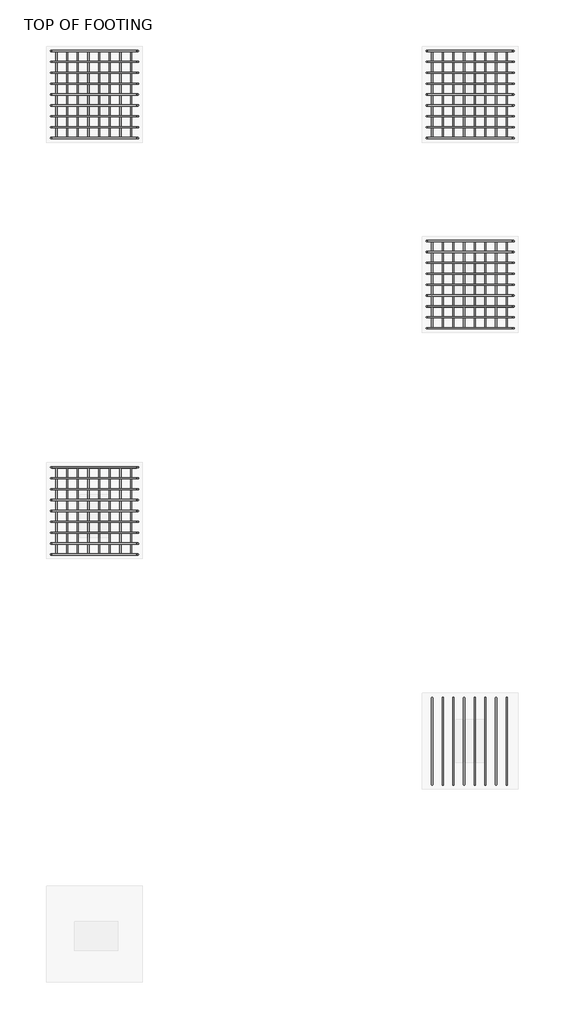
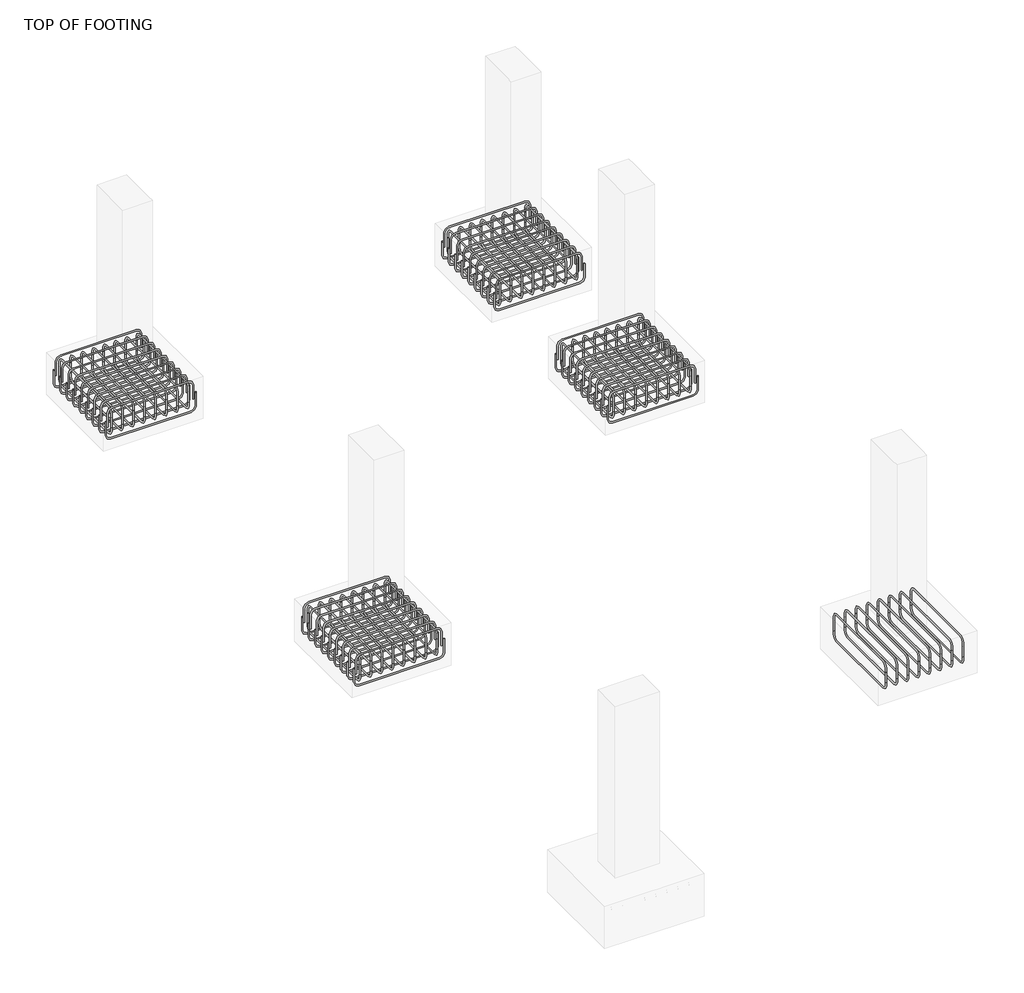
# One storey, part 12 of 20: 18 reinforcing bars.
"""IFC4 building model written with IfcOpenShell, lengths in millimetres."""

from ifc_helpers import new_model, si_unit, point, frame, origin, place, context, project, spatial, polyline, circle_curve, trimmed, segment, composite_curve, source, transform, mapped, element, save
from ifc_brep_helpers import swept_disk

model = new_model("IFC4")

# Units and contexts
model_context = context("Model", 3, world=origin())
ifc_project = project(units=[si_unit("LENGTHUNIT", "METRE", prefix="MILLI")], contexts=[model_context])

# Site, building, storey
site = spatial("IfcSite", under=ifc_project)
building = spatial("IfcBuilding", under=site)
storey = spatial("IfcBuildingStorey", under=building, Name="TOP OF FOOTING", Elevation=-1828.8)

# Reinforcing bars
placement = place(None, origin())
reinforcing_bar_shape = source(origin(), model_context, "Body", "SolidModel", [
    swept_disk(composite_curve([segment(polyline([(-5285.1605653, 14441.1679708, -2006.6587682), (-5285.1605653, 14441.1679708, -2153.9587682)]), True, "CONTINUOUS"), segment(trimmed(circle_curve(frame((-5331.5105653, 14441.1679708, -2153.9587682), z_axis=(0.0, 1.0, 0.0), x_axis=(46.350000000000364, 0.0, 0.0)), 46.35), [point((-5285.1605653, 14441.1679708, -2153.9587682))], [point((-5331.5105653, 14441.1679708, -2200.3087682))], True, "CARTESIAN"), True, "CONTINUOUS"), segment(polyline([(-5331.5105653, 14441.1679708, -2200.3087682), (-6146.1105653, 14441.1679708, -2200.3087682)]), True, "CONTINUOUS"), segment(trimmed(circle_curve(frame((-6146.1105653, 14441.1679708, -2153.9587682), z_axis=(0.0, 1.0, 0.0), x_axis=(0.0, 0.0, -46.34999999999991)), 46.35), [point((-6146.1105653, 14441.1679708, -2200.3087682))], [point((-6192.4605653, 14441.1679708, -2153.9587682))], True, "CARTESIAN"), True, "CONTINUOUS"), segment(polyline([(-6192.4605653, 14441.1679708, -2153.9587682), (-6192.4605653, 14441.1679708, -2006.6587682)]), True, "CONTINUOUS")], self_intersect=False), 6.35),
])
element("IfcReinforcingBar", 1, at=placement, inside=storey, context=model_context, shape_type="MappedRepresentation", body=[
    mapped(reinforcing_bar_shape, transform((0.0, 0.0, 0.0), x_axis=(1.0, 0.0, 0.0), y_axis=(0.0, 1.0, 0.0), z_axis=(0.0, 0.0, 1.0))),
    mapped(reinforcing_bar_shape, transform((0.0, -113.4125, 0.0), x_axis=(1.0, 0.0, 0.0), y_axis=(0.0, 1.0, 0.0), z_axis=(0.0, 0.0, 1.0))),
    mapped(reinforcing_bar_shape, transform((0.0, -226.825, 0.0), x_axis=(1.0, 0.0, 0.0), y_axis=(0.0, 1.0, 0.0), z_axis=(0.0, 0.0, 1.0))),
    mapped(reinforcing_bar_shape, transform((0.0, -340.2375, 0.0), x_axis=(1.0, 0.0, 0.0), y_axis=(0.0, 1.0, 0.0), z_axis=(0.0, 0.0, 1.0))),
    mapped(reinforcing_bar_shape, transform((0.0, -453.65, 0.0), x_axis=(1.0, 0.0, 0.0), y_axis=(0.0, 1.0, 0.0), z_axis=(0.0, 0.0, 1.0))),
    mapped(reinforcing_bar_shape, transform((0.0, -567.0625, 0.0), x_axis=(1.0, 0.0, 0.0), y_axis=(0.0, 1.0, 0.0), z_axis=(0.0, 0.0, 1.0))),
    mapped(reinforcing_bar_shape, transform((0.0, -680.475, 0.0), x_axis=(1.0, 0.0, 0.0), y_axis=(0.0, 1.0, 0.0), z_axis=(0.0, 0.0, 1.0))),
    mapped(reinforcing_bar_shape, transform((0.0, -793.8875, 0.0), x_axis=(1.0, 0.0, 0.0), y_axis=(0.0, 1.0, 0.0), z_axis=(0.0, 0.0, 1.0))),
    mapped(reinforcing_bar_shape, transform((0.0, -907.3, 0.0), x_axis=(1.0, 0.0, 0.0), y_axis=(0.0, 1.0, 0.0), z_axis=(0.0, 0.0, 1.0))),
])
reinforcing_bar_2_shape = source(origin(), model_context, "Body", "SolidModel", [
    swept_disk(composite_curve([segment(polyline([(-6172.986454, 14441.1679708, -2068.8), (-6172.986454, 14441.1679708, -1921.5)]), True, "CONTINUOUS"), segment(trimmed(circle_curve(frame((-6126.636454, 14441.1679708, -1921.5), z_axis=(0.0, 1.0, 0.0), x_axis=(-46.349999999999454, 0.0, 0.0)), 46.35), [point((-6172.986454, 14441.1679708, -1921.5))], [point((-6126.636454, 14441.1679708, -1875.15))], True, "CARTESIAN"), True, "CONTINUOUS"), segment(polyline([(-6126.636454, 14441.1679708, -1875.15), (-5357.1730543, 14441.1679708, -1875.15)]), True, "CONTINUOUS"), segment(trimmed(circle_curve(frame((-5357.1730543, 14441.1679708, -1921.5), z_axis=(0.0, 1.0, 0.0), x_axis=(0.0, 0.0, 46.34999999999991)), 46.35), [point((-5357.1730543, 14441.1679708, -1875.15))], [point((-5310.8230543, 14441.1679708, -1921.5))], True, "CARTESIAN"), True, "CONTINUOUS"), segment(polyline([(-5310.8230543, 14441.1679708, -1921.5), (-5310.8230543, 14441.1679708, -2068.8)]), True, "CONTINUOUS")], self_intersect=False), 6.35),
])
element("IfcReinforcingBar", 2, at=placement, inside=storey, context=model_context, shape_type="MappedRepresentation", body=[
    mapped(reinforcing_bar_2_shape, transform((0.0, 0.0, 0.0), x_axis=(1.0, 0.0, 0.0), y_axis=(0.0, 1.0, 0.0), z_axis=(0.0, 0.0, 1.0))),
    mapped(reinforcing_bar_2_shape, transform((0.0, -113.4125, 0.0), x_axis=(1.0, 0.0, 0.0), y_axis=(0.0, 1.0, 0.0), z_axis=(0.0, 0.0, 1.0))),
    mapped(reinforcing_bar_2_shape, transform((0.0, -226.825, 0.0), x_axis=(1.0, 0.0, 0.0), y_axis=(0.0, 1.0, 0.0), z_axis=(0.0, 0.0, 1.0))),
    mapped(reinforcing_bar_2_shape, transform((0.0, -340.2375, 0.0), x_axis=(1.0, 0.0, 0.0), y_axis=(0.0, 1.0, 0.0), z_axis=(0.0, 0.0, 1.0))),
    mapped(reinforcing_bar_2_shape, transform((0.0, -453.65, 0.0), x_axis=(1.0, 0.0, 0.0), y_axis=(0.0, 1.0, 0.0), z_axis=(0.0, 0.0, 1.0))),
    mapped(reinforcing_bar_2_shape, transform((0.0, -567.0625, 0.0), x_axis=(1.0, 0.0, 0.0), y_axis=(0.0, 1.0, 0.0), z_axis=(0.0, 0.0, 1.0))),
    mapped(reinforcing_bar_2_shape, transform((0.0, -680.475, 0.0), x_axis=(1.0, 0.0, 0.0), y_axis=(0.0, 1.0, 0.0), z_axis=(0.0, 0.0, 1.0))),
    mapped(reinforcing_bar_2_shape, transform((0.0, -793.8875, 0.0), x_axis=(1.0, 0.0, 0.0), y_axis=(0.0, 1.0, 0.0), z_axis=(0.0, 0.0, 1.0))),
    mapped(reinforcing_bar_2_shape, transform((0.0, -907.3, 0.0), x_axis=(1.0, 0.0, 0.0), y_axis=(0.0, 1.0, 0.0), z_axis=(0.0, 0.0, 1.0))),
])
reinforcing_bar_3_shape = source(origin(), model_context, "Body", "SolidModel", [
    swept_disk(composite_curve([segment(polyline([(-5356.6575267, 14441.1679708, -2086.1951968), (-5356.6575267, 14441.1679708, -1938.8951968)]), True, "CONTINUOUS"), segment(trimmed(circle_curve(frame((-5356.6575267, 14394.8179708, -1938.8951968), z_axis=(1.0, 0.0, 0.0), x_axis=(0.0, 46.349999999998545, 0.0)), 46.35), [point((-5356.6575267, 14441.1679708, -1938.8951968))], [point((-5356.6575267, 14394.8179708, -1892.5451968))], True, "CARTESIAN"), True, "CONTINUOUS"), segment(polyline([(-5356.6575267, 14394.8179708, -1892.5451968), (-5356.6575267, 13580.2179708, -1892.5451968)]), True, "CONTINUOUS"), segment(trimmed(circle_curve(frame((-5356.6575267, 13580.2179708, -1938.8951968), z_axis=(1.0, 0.0, 0.0), x_axis=(0.0, 0.0, 46.34999999999991)), 46.35), [point((-5356.6575267, 13580.2179708, -1892.5451968))], [point((-5356.6575267, 13533.8679708, -1938.8951968))], True, "CARTESIAN"), True, "CONTINUOUS"), segment(polyline([(-5356.6575267, 13533.8679708, -1938.8951968), (-5356.6575267, 13533.8679708, -2086.1951968)]), True, "CONTINUOUS")], self_intersect=False), 6.35),
])
element("IfcReinforcingBar", 3, at=placement, inside=storey, context=model_context, shape_type="MappedRepresentation", body=[
    mapped(reinforcing_bar_3_shape, transform((0.0, 0.0, 0.0), x_axis=(1.0, 0.0, 0.0), y_axis=(0.0, 1.0, 0.0), z_axis=(0.0, 0.0, 1.0))),
    mapped(reinforcing_bar_3_shape, transform((-111.2862402, 0.0, 0.0), x_axis=(1.0, 0.0, 0.0), y_axis=(0.0, 1.0, 0.0), z_axis=(0.0, 0.0, 1.0))),
    mapped(reinforcing_bar_3_shape, transform((-222.5724804, 0.0, 0.0), x_axis=(1.0, 0.0, 0.0), y_axis=(0.0, 1.0, 0.0), z_axis=(0.0, 0.0, 1.0))),
    mapped(reinforcing_bar_3_shape, transform((-333.8587205, 0.0, 0.0), x_axis=(1.0, 0.0, 0.0), y_axis=(0.0, 1.0, 0.0), z_axis=(0.0, 0.0, 1.0))),
    mapped(reinforcing_bar_3_shape, transform((-445.1449607, 0.0, 0.0), x_axis=(1.0, 0.0, 0.0), y_axis=(0.0, 1.0, 0.0), z_axis=(0.0, 0.0, 1.0))),
    mapped(reinforcing_bar_3_shape, transform((-556.4312009, 0.0, 0.0), x_axis=(1.0, 0.0, 0.0), y_axis=(0.0, 1.0, 0.0), z_axis=(0.0, 0.0, 1.0))),
    mapped(reinforcing_bar_3_shape, transform((-667.7174411, 0.0, 0.0), x_axis=(1.0, 0.0, 0.0), y_axis=(0.0, 1.0, 0.0), z_axis=(0.0, 0.0, 1.0))),
    mapped(reinforcing_bar_3_shape, transform((-779.0036813, 0.0, 0.0), x_axis=(1.0, 0.0, 0.0), y_axis=(0.0, 1.0, 0.0), z_axis=(0.0, 0.0, 1.0))),
])
reinforcing_bar_4_shape = source(origin(), model_context, "Body", "SolidModel", [
    swept_disk(composite_curve([segment(polyline([(-6135.661208, 14441.1679708, -1979.1645013), (-6135.661208, 14441.1679708, -2126.4645013)]), True, "CONTINUOUS"), segment(trimmed(circle_curve(frame((-6135.661208, 14394.8179708, -2126.4645013), z_axis=(-1.0, 0.0, 0.0), x_axis=(0.0, 46.349999999998545, 0.0)), 46.35), [point((-6135.661208, 14441.1679708, -2126.4645013))], [point((-6135.661208, 14394.8179708, -2172.8145013))], True, "CARTESIAN"), True, "CONTINUOUS"), segment(polyline([(-6135.661208, 14394.8179708, -2172.8145013), (-6135.661208, 13580.2179708, -2172.8145013)]), True, "CONTINUOUS"), segment(trimmed(circle_curve(frame((-6135.661208, 13580.2179708, -2126.4645013), z_axis=(-1.0, 0.0, 0.0), x_axis=(0.0, 0.0, -46.34999999999991)), 46.35), [point((-6135.661208, 13580.2179708, -2172.8145013))], [point((-6135.661208, 13533.8679708, -2126.4645013))], True, "CARTESIAN"), True, "CONTINUOUS"), segment(polyline([(-6135.661208, 13533.8679708, -2126.4645013), (-6135.661208, 13533.8679708, -1979.1645013)]), True, "CONTINUOUS")], self_intersect=False), 6.35),
])
element("IfcReinforcingBar", 4, at=placement, inside=storey, context=model_context, shape_type="MappedRepresentation", body=[
    mapped(reinforcing_bar_4_shape, transform((0.0, 0.0, 0.0), x_axis=(1.0, 0.0, 0.0), y_axis=(0.0, 1.0, 0.0), z_axis=(0.0, 0.0, 1.0))),
    mapped(reinforcing_bar_4_shape, transform((111.2862402, 0.0, 0.0), x_axis=(1.0, 0.0, 0.0), y_axis=(0.0, 1.0, 0.0), z_axis=(0.0, 0.0, 1.0))),
    mapped(reinforcing_bar_4_shape, transform((222.5724804, 0.0, 0.0), x_axis=(1.0, 0.0, 0.0), y_axis=(0.0, 1.0, 0.0), z_axis=(0.0, 0.0, 1.0))),
    mapped(reinforcing_bar_4_shape, transform((333.8587205, 0.0, 0.0), x_axis=(1.0, 0.0, 0.0), y_axis=(0.0, 1.0, 0.0), z_axis=(0.0, 0.0, 1.0))),
    mapped(reinforcing_bar_4_shape, transform((445.1449607, 0.0, 0.0), x_axis=(1.0, 0.0, 0.0), y_axis=(0.0, 1.0, 0.0), z_axis=(0.0, 0.0, 1.0))),
    mapped(reinforcing_bar_4_shape, transform((556.4312009, 0.0, 0.0), x_axis=(1.0, 0.0, 0.0), y_axis=(0.0, 1.0, 0.0), z_axis=(0.0, 0.0, 1.0))),
    mapped(reinforcing_bar_4_shape, transform((667.7174411, 0.0, 0.0), x_axis=(1.0, 0.0, 0.0), y_axis=(0.0, 1.0, 0.0), z_axis=(0.0, 0.0, 1.0))),
    mapped(reinforcing_bar_4_shape, transform((779.0036813, 0.0, 0.0), x_axis=(1.0, 0.0, 0.0), y_axis=(0.0, 1.0, 0.0), z_axis=(0.0, 0.0, 1.0))),
])
reinforcing_bar_5_shape = source(origin(), model_context, "Body", "SolidModel", [
    swept_disk(composite_curve([segment(polyline([(-5285.1605653, 10103.3576276, -2006.6587682), (-5285.1605653, 10103.3576276, -2153.9587682)]), True, "CONTINUOUS"), segment(trimmed(circle_curve(frame((-5331.5105653, 10103.3576276, -2153.9587682), z_axis=(0.0, 1.0, 0.0), x_axis=(46.350000000000364, 0.0, 0.0)), 46.35), [point((-5285.1605653, 10103.3576276, -2153.9587682))], [point((-5331.5105653, 10103.3576276, -2200.3087682))], True, "CARTESIAN"), True, "CONTINUOUS"), segment(polyline([(-5331.5105653, 10103.3576276, -2200.3087682), (-6146.1105653, 10103.3576276, -2200.3087682)]), True, "CONTINUOUS"), segment(trimmed(circle_curve(frame((-6146.1105653, 10103.3576276, -2153.9587682), z_axis=(0.0, 1.0, 0.0), x_axis=(0.0, 0.0, -46.34999999999991)), 46.35), [point((-6146.1105653, 10103.3576276, -2200.3087682))], [point((-6192.4605653, 10103.3576276, -2153.9587682))], True, "CARTESIAN"), True, "CONTINUOUS"), segment(polyline([(-6192.4605653, 10103.3576276, -2153.9587682), (-6192.4605653, 10103.3576276, -2006.6587682)]), True, "CONTINUOUS")], self_intersect=False), 6.35),
])
element("IfcReinforcingBar", 5, at=placement, inside=storey, context=model_context, shape_type="MappedRepresentation", body=[
    mapped(reinforcing_bar_5_shape, transform((0.0, 0.0, 0.0), x_axis=(1.0, 0.0, 0.0), y_axis=(0.0, 1.0, 0.0), z_axis=(0.0, 0.0, 1.0))),
    mapped(reinforcing_bar_5_shape, transform((0.0, -113.4125, 0.0), x_axis=(1.0, 0.0, 0.0), y_axis=(0.0, 1.0, 0.0), z_axis=(0.0, 0.0, 1.0))),
    mapped(reinforcing_bar_5_shape, transform((0.0, -226.825, 0.0), x_axis=(1.0, 0.0, 0.0), y_axis=(0.0, 1.0, 0.0), z_axis=(0.0, 0.0, 1.0))),
    mapped(reinforcing_bar_5_shape, transform((0.0, -340.2375, 0.0), x_axis=(1.0, 0.0, 0.0), y_axis=(0.0, 1.0, 0.0), z_axis=(0.0, 0.0, 1.0))),
    mapped(reinforcing_bar_5_shape, transform((0.0, -453.65, 0.0), x_axis=(1.0, 0.0, 0.0), y_axis=(0.0, 1.0, 0.0), z_axis=(0.0, 0.0, 1.0))),
    mapped(reinforcing_bar_5_shape, transform((0.0, -567.0625, 0.0), x_axis=(1.0, 0.0, 0.0), y_axis=(0.0, 1.0, 0.0), z_axis=(0.0, 0.0, 1.0))),
    mapped(reinforcing_bar_5_shape, transform((0.0, -680.475, 0.0), x_axis=(1.0, 0.0, 0.0), y_axis=(0.0, 1.0, 0.0), z_axis=(0.0, 0.0, 1.0))),
    mapped(reinforcing_bar_5_shape, transform((0.0, -793.8875, 0.0), x_axis=(1.0, 0.0, 0.0), y_axis=(0.0, 1.0, 0.0), z_axis=(0.0, 0.0, 1.0))),
    mapped(reinforcing_bar_5_shape, transform((0.0, -907.3, 0.0), x_axis=(1.0, 0.0, 0.0), y_axis=(0.0, 1.0, 0.0), z_axis=(0.0, 0.0, 1.0))),
])
reinforcing_bar_6_shape = source(origin(), model_context, "Body", "SolidModel", [
    swept_disk(composite_curve([segment(polyline([(-6172.986454, 10103.3576276, -2068.8), (-6172.986454, 10103.3576276, -1921.5)]), True, "CONTINUOUS"), segment(trimmed(circle_curve(frame((-6126.636454, 10103.3576276, -1921.5), z_axis=(0.0, 1.0, 0.0), x_axis=(-46.349999999999454, 0.0, 0.0)), 46.35), [point((-6172.986454, 10103.3576276, -1921.5))], [point((-6126.636454, 10103.3576276, -1875.15))], True, "CARTESIAN"), True, "CONTINUOUS"), segment(polyline([(-6126.636454, 10103.3576276, -1875.15), (-5357.1730543, 10103.3576276, -1875.15)]), True, "CONTINUOUS"), segment(trimmed(circle_curve(frame((-5357.1730543, 10103.3576276, -1921.5), z_axis=(0.0, 1.0, 0.0), x_axis=(0.0, 0.0, 46.34999999999991)), 46.35), [point((-5357.1730543, 10103.3576276, -1875.15))], [point((-5310.8230543, 10103.3576276, -1921.5))], True, "CARTESIAN"), True, "CONTINUOUS"), segment(polyline([(-5310.8230543, 10103.3576276, -1921.5), (-5310.8230543, 10103.3576276, -2068.8)]), True, "CONTINUOUS")], self_intersect=False), 6.35),
])
element("IfcReinforcingBar", 6, at=placement, inside=storey, context=model_context, shape_type="MappedRepresentation", body=[
    mapped(reinforcing_bar_6_shape, transform((0.0, 0.0, 0.0), x_axis=(1.0, 0.0, 0.0), y_axis=(0.0, 1.0, 0.0), z_axis=(0.0, 0.0, 1.0))),
    mapped(reinforcing_bar_6_shape, transform((0.0, -113.4125, 0.0), x_axis=(1.0, 0.0, 0.0), y_axis=(0.0, 1.0, 0.0), z_axis=(0.0, 0.0, 1.0))),
    mapped(reinforcing_bar_6_shape, transform((0.0, -226.825, 0.0), x_axis=(1.0, 0.0, 0.0), y_axis=(0.0, 1.0, 0.0), z_axis=(0.0, 0.0, 1.0))),
    mapped(reinforcing_bar_6_shape, transform((0.0, -340.2375, 0.0), x_axis=(1.0, 0.0, 0.0), y_axis=(0.0, 1.0, 0.0), z_axis=(0.0, 0.0, 1.0))),
    mapped(reinforcing_bar_6_shape, transform((0.0, -453.65, 0.0), x_axis=(1.0, 0.0, 0.0), y_axis=(0.0, 1.0, 0.0), z_axis=(0.0, 0.0, 1.0))),
    mapped(reinforcing_bar_6_shape, transform((0.0, -567.0625, 0.0), x_axis=(1.0, 0.0, 0.0), y_axis=(0.0, 1.0, 0.0), z_axis=(0.0, 0.0, 1.0))),
    mapped(reinforcing_bar_6_shape, transform((0.0, -680.475, 0.0), x_axis=(1.0, 0.0, 0.0), y_axis=(0.0, 1.0, 0.0), z_axis=(0.0, 0.0, 1.0))),
    mapped(reinforcing_bar_6_shape, transform((0.0, -793.8875, 0.0), x_axis=(1.0, 0.0, 0.0), y_axis=(0.0, 1.0, 0.0), z_axis=(0.0, 0.0, 1.0))),
    mapped(reinforcing_bar_6_shape, transform((0.0, -907.3, 0.0), x_axis=(1.0, 0.0, 0.0), y_axis=(0.0, 1.0, 0.0), z_axis=(0.0, 0.0, 1.0))),
])
reinforcing_bar_7_shape = source(origin(), model_context, "Body", "SolidModel", [
    swept_disk(composite_curve([segment(polyline([(-5356.6575267, 10103.3576276, -2086.1951968), (-5356.6575267, 10103.3576276, -1938.8951968)]), True, "CONTINUOUS"), segment(trimmed(circle_curve(frame((-5356.6575267, 10057.0076276, -1938.8951968), z_axis=(1.0, 0.0, 0.0), x_axis=(0.0, 46.350000000000364, 0.0)), 46.35), [point((-5356.6575267, 10103.3576276, -1938.8951968))], [point((-5356.6575267, 10057.0076276, -1892.5451968))], True, "CARTESIAN"), True, "CONTINUOUS"), segment(polyline([(-5356.6575267, 10057.0076276, -1892.5451968), (-5356.6575267, 9242.4076276, -1892.5451968)]), True, "CONTINUOUS"), segment(trimmed(circle_curve(frame((-5356.6575267, 9242.4076276, -1938.8951968), z_axis=(1.0, 0.0, 0.0), x_axis=(0.0, 0.0, 46.34999999999991)), 46.35), [point((-5356.6575267, 9242.4076276, -1892.5451968))], [point((-5356.6575267, 9196.0576276, -1938.8951968))], True, "CARTESIAN"), True, "CONTINUOUS"), segment(polyline([(-5356.6575267, 9196.0576276, -1938.8951968), (-5356.6575267, 9196.0576276, -2086.1951968)]), True, "CONTINUOUS")], self_intersect=False), 6.35),
])
element("IfcReinforcingBar", 7, at=placement, inside=storey, context=model_context, shape_type="MappedRepresentation", body=[
    mapped(reinforcing_bar_7_shape, transform((0.0, 0.0, 0.0), x_axis=(1.0, 0.0, 0.0), y_axis=(0.0, 1.0, 0.0), z_axis=(0.0, 0.0, 1.0))),
    mapped(reinforcing_bar_7_shape, transform((-111.2862402, 0.0, 0.0), x_axis=(1.0, 0.0, 0.0), y_axis=(0.0, 1.0, 0.0), z_axis=(0.0, 0.0, 1.0))),
    mapped(reinforcing_bar_7_shape, transform((-222.5724804, 0.0, 0.0), x_axis=(1.0, 0.0, 0.0), y_axis=(0.0, 1.0, 0.0), z_axis=(0.0, 0.0, 1.0))),
    mapped(reinforcing_bar_7_shape, transform((-333.8587205, 0.0, 0.0), x_axis=(1.0, 0.0, 0.0), y_axis=(0.0, 1.0, 0.0), z_axis=(0.0, 0.0, 1.0))),
    mapped(reinforcing_bar_7_shape, transform((-445.1449607, 0.0, 0.0), x_axis=(1.0, 0.0, 0.0), y_axis=(0.0, 1.0, 0.0), z_axis=(0.0, 0.0, 1.0))),
    mapped(reinforcing_bar_7_shape, transform((-556.4312009, 0.0, 0.0), x_axis=(1.0, 0.0, 0.0), y_axis=(0.0, 1.0, 0.0), z_axis=(0.0, 0.0, 1.0))),
    mapped(reinforcing_bar_7_shape, transform((-667.7174411, 0.0, 0.0), x_axis=(1.0, 0.0, 0.0), y_axis=(0.0, 1.0, 0.0), z_axis=(0.0, 0.0, 1.0))),
    mapped(reinforcing_bar_7_shape, transform((-779.0036813, 0.0, 0.0), x_axis=(1.0, 0.0, 0.0), y_axis=(0.0, 1.0, 0.0), z_axis=(0.0, 0.0, 1.0))),
])
reinforcing_bar_8_shape = source(origin(), model_context, "Body", "SolidModel", [
    swept_disk(composite_curve([segment(polyline([(-6135.661208, 10103.3576276, -1979.1645013), (-6135.661208, 10103.3576276, -2126.4645013)]), True, "CONTINUOUS"), segment(trimmed(circle_curve(frame((-6135.661208, 10057.0076276, -2126.4645013), z_axis=(-1.0, 0.0, 0.0), x_axis=(0.0, 46.350000000000364, 0.0)), 46.35), [point((-6135.661208, 10103.3576276, -2126.4645013))], [point((-6135.661208, 10057.0076276, -2172.8145013))], True, "CARTESIAN"), True, "CONTINUOUS"), segment(polyline([(-6135.661208, 10057.0076276, -2172.8145013), (-6135.661208, 9242.4076276, -2172.8145013)]), True, "CONTINUOUS"), segment(trimmed(circle_curve(frame((-6135.661208, 9242.4076276, -2126.4645013), z_axis=(-1.0, 0.0, 0.0), x_axis=(0.0, 0.0, -46.34999999999991)), 46.35), [point((-6135.661208, 9242.4076276, -2172.8145013))], [point((-6135.661208, 9196.0576276, -2126.4645013))], True, "CARTESIAN"), True, "CONTINUOUS"), segment(polyline([(-6135.661208, 9196.0576276, -2126.4645013), (-6135.661208, 9196.0576276, -1979.1645013)]), True, "CONTINUOUS")], self_intersect=False), 6.35),
])
element("IfcReinforcingBar", 8, at=placement, inside=storey, context=model_context, shape_type="MappedRepresentation", body=[
    mapped(reinforcing_bar_8_shape, transform((0.0, 0.0, 0.0), x_axis=(1.0, 0.0, 0.0), y_axis=(0.0, 1.0, 0.0), z_axis=(0.0, 0.0, 1.0))),
    mapped(reinforcing_bar_8_shape, transform((111.2862402, 0.0, 0.0), x_axis=(1.0, 0.0, 0.0), y_axis=(0.0, 1.0, 0.0), z_axis=(0.0, 0.0, 1.0))),
    mapped(reinforcing_bar_8_shape, transform((222.5724804, 0.0, 0.0), x_axis=(1.0, 0.0, 0.0), y_axis=(0.0, 1.0, 0.0), z_axis=(0.0, 0.0, 1.0))),
    mapped(reinforcing_bar_8_shape, transform((333.8587205, 0.0, 0.0), x_axis=(1.0, 0.0, 0.0), y_axis=(0.0, 1.0, 0.0), z_axis=(0.0, 0.0, 1.0))),
    mapped(reinforcing_bar_8_shape, transform((445.1449607, 0.0, 0.0), x_axis=(1.0, 0.0, 0.0), y_axis=(0.0, 1.0, 0.0), z_axis=(0.0, 0.0, 1.0))),
    mapped(reinforcing_bar_8_shape, transform((556.4312009, 0.0, 0.0), x_axis=(1.0, 0.0, 0.0), y_axis=(0.0, 1.0, 0.0), z_axis=(0.0, 0.0, 1.0))),
    mapped(reinforcing_bar_8_shape, transform((667.7174411, 0.0, 0.0), x_axis=(1.0, 0.0, 0.0), y_axis=(0.0, 1.0, 0.0), z_axis=(0.0, 0.0, 1.0))),
    mapped(reinforcing_bar_8_shape, transform((779.0036813, 0.0, 0.0), x_axis=(1.0, 0.0, 0.0), y_axis=(0.0, 1.0, 0.0), z_axis=(0.0, 0.0, 1.0))),
])
reinforcing_bar_9_shape = source(origin(), model_context, "Body", "SolidModel", [
    swept_disk(composite_curve([segment(polyline([(-1368.1365686, 14441.1679708, -2006.6587682), (-1368.1365686, 14441.1679708, -2153.9587682)]), True, "CONTINUOUS"), segment(trimmed(circle_curve(frame((-1414.4865686, 14441.1679708, -2153.9587682), z_axis=(0.0, 1.0, 0.0), x_axis=(46.350000000000136, 0.0, 0.0)), 46.35), [point((-1368.1365686, 14441.1679708, -2153.9587682))], [point((-1414.4865686, 14441.1679708, -2200.3087682))], True, "CARTESIAN"), True, "CONTINUOUS"), segment(polyline([(-1414.4865686, 14441.1679708, -2200.3087682), (-2229.0865686, 14441.1679708, -2200.3087682)]), True, "CONTINUOUS"), segment(trimmed(circle_curve(frame((-2229.0865686, 14441.1679708, -2153.9587682), z_axis=(0.0, 1.0, 0.0), x_axis=(0.0, 0.0, -46.34999999999991)), 46.35), [point((-2229.0865686, 14441.1679708, -2200.3087682))], [point((-2275.4365686, 14441.1679708, -2153.9587682))], True, "CARTESIAN"), True, "CONTINUOUS"), segment(polyline([(-2275.4365686, 14441.1679708, -2153.9587682), (-2275.4365686, 14441.1679708, -2006.6587682)]), True, "CONTINUOUS")], self_intersect=False), 6.35),
])
element("IfcReinforcingBar", 9, at=placement, inside=storey, context=model_context, shape_type="MappedRepresentation", body=[
    mapped(reinforcing_bar_9_shape, transform((0.0, 0.0, 0.0), x_axis=(1.0, 0.0, 0.0), y_axis=(0.0, 1.0, 0.0), z_axis=(0.0, 0.0, 1.0))),
    mapped(reinforcing_bar_9_shape, transform((0.0, -113.4125, 0.0), x_axis=(1.0, 0.0, 0.0), y_axis=(0.0, 1.0, 0.0), z_axis=(0.0, 0.0, 1.0))),
    mapped(reinforcing_bar_9_shape, transform((0.0, -226.825, 0.0), x_axis=(1.0, 0.0, 0.0), y_axis=(0.0, 1.0, 0.0), z_axis=(0.0, 0.0, 1.0))),
    mapped(reinforcing_bar_9_shape, transform((0.0, -340.2375, 0.0), x_axis=(1.0, 0.0, 0.0), y_axis=(0.0, 1.0, 0.0), z_axis=(0.0, 0.0, 1.0))),
    mapped(reinforcing_bar_9_shape, transform((0.0, -453.65, 0.0), x_axis=(1.0, 0.0, 0.0), y_axis=(0.0, 1.0, 0.0), z_axis=(0.0, 0.0, 1.0))),
    mapped(reinforcing_bar_9_shape, transform((0.0, -567.0625, 0.0), x_axis=(1.0, 0.0, 0.0), y_axis=(0.0, 1.0, 0.0), z_axis=(0.0, 0.0, 1.0))),
    mapped(reinforcing_bar_9_shape, transform((0.0, -680.475, 0.0), x_axis=(1.0, 0.0, 0.0), y_axis=(0.0, 1.0, 0.0), z_axis=(0.0, 0.0, 1.0))),
    mapped(reinforcing_bar_9_shape, transform((0.0, -793.8875, 0.0), x_axis=(1.0, 0.0, 0.0), y_axis=(0.0, 1.0, 0.0), z_axis=(0.0, 0.0, 1.0))),
    mapped(reinforcing_bar_9_shape, transform((0.0, -907.3, 0.0), x_axis=(1.0, 0.0, 0.0), y_axis=(0.0, 1.0, 0.0), z_axis=(0.0, 0.0, 1.0))),
])
reinforcing_bar_10_shape = source(origin(), model_context, "Body", "SolidModel", [
    swept_disk(composite_curve([segment(polyline([(-2255.9624573, 14441.1679708, -2068.8), (-2255.9624573, 14441.1679708, -1921.5)]), True, "CONTINUOUS"), segment(trimmed(circle_curve(frame((-2209.6124573, 14441.1679708, -1921.5), z_axis=(0.0, 1.0, 0.0), x_axis=(-46.34999999999991, 0.0, 0.0)), 46.35), [point((-2255.9624573, 14441.1679708, -1921.5))], [point((-2209.6124573, 14441.1679708, -1875.15))], True, "CARTESIAN"), True, "CONTINUOUS"), segment(polyline([(-2209.6124573, 14441.1679708, -1875.15), (-1440.1490576, 14441.1679708, -1875.15)]), True, "CONTINUOUS"), segment(trimmed(circle_curve(frame((-1440.1490576, 14441.1679708, -1921.5), z_axis=(0.0, 1.0, 0.0), x_axis=(0.0, 0.0, 46.34999999999991)), 46.35), [point((-1440.1490576, 14441.1679708, -1875.15))], [point((-1393.7990576, 14441.1679708, -1921.5))], True, "CARTESIAN"), True, "CONTINUOUS"), segment(polyline([(-1393.7990576, 14441.1679708, -1921.5), (-1393.7990576, 14441.1679708, -2068.8)]), True, "CONTINUOUS")], self_intersect=False), 6.35),
])
element("IfcReinforcingBar", 10, at=placement, inside=storey, context=model_context, shape_type="MappedRepresentation", body=[
    mapped(reinforcing_bar_10_shape, transform((0.0, 0.0, 0.0), x_axis=(1.0, 0.0, 0.0), y_axis=(0.0, 1.0, 0.0), z_axis=(0.0, 0.0, 1.0))),
    mapped(reinforcing_bar_10_shape, transform((0.0, -113.4125, 0.0), x_axis=(1.0, 0.0, 0.0), y_axis=(0.0, 1.0, 0.0), z_axis=(0.0, 0.0, 1.0))),
    mapped(reinforcing_bar_10_shape, transform((0.0, -226.825, 0.0), x_axis=(1.0, 0.0, 0.0), y_axis=(0.0, 1.0, 0.0), z_axis=(0.0, 0.0, 1.0))),
    mapped(reinforcing_bar_10_shape, transform((0.0, -340.2375, 0.0), x_axis=(1.0, 0.0, 0.0), y_axis=(0.0, 1.0, 0.0), z_axis=(0.0, 0.0, 1.0))),
    mapped(reinforcing_bar_10_shape, transform((0.0, -453.65, 0.0), x_axis=(1.0, 0.0, 0.0), y_axis=(0.0, 1.0, 0.0), z_axis=(0.0, 0.0, 1.0))),
    mapped(reinforcing_bar_10_shape, transform((0.0, -567.0625, 0.0), x_axis=(1.0, 0.0, 0.0), y_axis=(0.0, 1.0, 0.0), z_axis=(0.0, 0.0, 1.0))),
    mapped(reinforcing_bar_10_shape, transform((0.0, -680.475, 0.0), x_axis=(1.0, 0.0, 0.0), y_axis=(0.0, 1.0, 0.0), z_axis=(0.0, 0.0, 1.0))),
    mapped(reinforcing_bar_10_shape, transform((0.0, -793.8875, 0.0), x_axis=(1.0, 0.0, 0.0), y_axis=(0.0, 1.0, 0.0), z_axis=(0.0, 0.0, 1.0))),
    mapped(reinforcing_bar_10_shape, transform((0.0, -907.3, 0.0), x_axis=(1.0, 0.0, 0.0), y_axis=(0.0, 1.0, 0.0), z_axis=(0.0, 0.0, 1.0))),
])
reinforcing_bar_11_shape = source(origin(), model_context, "Body", "SolidModel", [
    swept_disk(composite_curve([segment(polyline([(-1439.63353, 14441.1679708, -2086.1951968), (-1439.63353, 14441.1679708, -1938.8951968)]), True, "CONTINUOUS"), segment(trimmed(circle_curve(frame((-1439.63353, 14394.8179708, -1938.8951968), z_axis=(1.0, 0.0, 0.0), x_axis=(0.0, 46.349999999998545, 0.0)), 46.35), [point((-1439.63353, 14441.1679708, -1938.8951968))], [point((-1439.63353, 14394.8179708, -1892.5451968))], True, "CARTESIAN"), True, "CONTINUOUS"), segment(polyline([(-1439.63353, 14394.8179708, -1892.5451968), (-1439.63353, 13580.2179708, -1892.5451968)]), True, "CONTINUOUS"), segment(trimmed(circle_curve(frame((-1439.63353, 13580.2179708, -1938.8951968), z_axis=(1.0, 0.0, 0.0), x_axis=(0.0, 0.0, 46.34999999999991)), 46.35), [point((-1439.63353, 13580.2179708, -1892.5451968))], [point((-1439.63353, 13533.8679708, -1938.8951968))], True, "CARTESIAN"), True, "CONTINUOUS"), segment(polyline([(-1439.63353, 13533.8679708, -1938.8951968), (-1439.63353, 13533.8679708, -2086.1951968)]), True, "CONTINUOUS")], self_intersect=False), 6.35),
])
element("IfcReinforcingBar", 11, at=placement, inside=storey, context=model_context, shape_type="MappedRepresentation", body=[
    mapped(reinforcing_bar_11_shape, transform((0.0, 0.0, 0.0), x_axis=(1.0, 0.0, 0.0), y_axis=(0.0, 1.0, 0.0), z_axis=(0.0, 0.0, 1.0))),
    mapped(reinforcing_bar_11_shape, transform((-111.2862402, 0.0, 0.0), x_axis=(1.0, 0.0, 0.0), y_axis=(0.0, 1.0, 0.0), z_axis=(0.0, 0.0, 1.0))),
    mapped(reinforcing_bar_11_shape, transform((-222.5724804, 0.0, 0.0), x_axis=(1.0, 0.0, 0.0), y_axis=(0.0, 1.0, 0.0), z_axis=(0.0, 0.0, 1.0))),
    mapped(reinforcing_bar_11_shape, transform((-333.8587205, 0.0, 0.0), x_axis=(1.0, 0.0, 0.0), y_axis=(0.0, 1.0, 0.0), z_axis=(0.0, 0.0, 1.0))),
    mapped(reinforcing_bar_11_shape, transform((-445.1449607, 0.0, 0.0), x_axis=(1.0, 0.0, 0.0), y_axis=(0.0, 1.0, 0.0), z_axis=(0.0, 0.0, 1.0))),
    mapped(reinforcing_bar_11_shape, transform((-556.4312009, 0.0, 0.0), x_axis=(1.0, 0.0, 0.0), y_axis=(0.0, 1.0, 0.0), z_axis=(0.0, 0.0, 1.0))),
    mapped(reinforcing_bar_11_shape, transform((-667.7174411, 0.0, 0.0), x_axis=(1.0, 0.0, 0.0), y_axis=(0.0, 1.0, 0.0), z_axis=(0.0, 0.0, 1.0))),
    mapped(reinforcing_bar_11_shape, transform((-779.0036813, 0.0, 0.0), x_axis=(1.0, 0.0, 0.0), y_axis=(0.0, 1.0, 0.0), z_axis=(0.0, 0.0, 1.0))),
])
reinforcing_bar_12_shape = source(origin(), model_context, "Body", "SolidModel", [
    swept_disk(composite_curve([segment(polyline([(-2218.6372113, 14441.1679708, -1979.1645013), (-2218.6372113, 14441.1679708, -2126.4645013)]), True, "CONTINUOUS"), segment(trimmed(circle_curve(frame((-2218.6372113, 14394.8179708, -2126.4645013), z_axis=(-1.0, 0.0, 0.0), x_axis=(0.0, 46.349999999998545, 0.0)), 46.35), [point((-2218.6372113, 14441.1679708, -2126.4645013))], [point((-2218.6372113, 14394.8179708, -2172.8145013))], True, "CARTESIAN"), True, "CONTINUOUS"), segment(polyline([(-2218.6372113, 14394.8179708, -2172.8145013), (-2218.6372113, 13580.2179708, -2172.8145013)]), True, "CONTINUOUS"), segment(trimmed(circle_curve(frame((-2218.6372113, 13580.2179708, -2126.4645013), z_axis=(-1.0, 0.0, 0.0), x_axis=(0.0, 0.0, -46.34999999999991)), 46.35), [point((-2218.6372113, 13580.2179708, -2172.8145013))], [point((-2218.6372113, 13533.8679708, -2126.4645013))], True, "CARTESIAN"), True, "CONTINUOUS"), segment(polyline([(-2218.6372113, 13533.8679708, -2126.4645013), (-2218.6372113, 13533.8679708, -1979.1645013)]), True, "CONTINUOUS")], self_intersect=False), 6.35),
])
element("IfcReinforcingBar", 12, at=placement, inside=storey, context=model_context, shape_type="MappedRepresentation", body=[
    mapped(reinforcing_bar_12_shape, transform((0.0, 0.0, 0.0), x_axis=(1.0, 0.0, 0.0), y_axis=(0.0, 1.0, 0.0), z_axis=(0.0, 0.0, 1.0))),
    mapped(reinforcing_bar_12_shape, transform((111.2862402, 0.0, 0.0), x_axis=(1.0, 0.0, 0.0), y_axis=(0.0, 1.0, 0.0), z_axis=(0.0, 0.0, 1.0))),
    mapped(reinforcing_bar_12_shape, transform((222.5724804, 0.0, 0.0), x_axis=(1.0, 0.0, 0.0), y_axis=(0.0, 1.0, 0.0), z_axis=(0.0, 0.0, 1.0))),
    mapped(reinforcing_bar_12_shape, transform((333.8587205, 0.0, 0.0), x_axis=(1.0, 0.0, 0.0), y_axis=(0.0, 1.0, 0.0), z_axis=(0.0, 0.0, 1.0))),
    mapped(reinforcing_bar_12_shape, transform((445.1449607, 0.0, 0.0), x_axis=(1.0, 0.0, 0.0), y_axis=(0.0, 1.0, 0.0), z_axis=(0.0, 0.0, 1.0))),
    mapped(reinforcing_bar_12_shape, transform((556.4312009, 0.0, 0.0), x_axis=(1.0, 0.0, 0.0), y_axis=(0.0, 1.0, 0.0), z_axis=(0.0, 0.0, 1.0))),
    mapped(reinforcing_bar_12_shape, transform((667.7174411, 0.0, 0.0), x_axis=(1.0, 0.0, 0.0), y_axis=(0.0, 1.0, 0.0), z_axis=(0.0, 0.0, 1.0))),
    mapped(reinforcing_bar_12_shape, transform((779.0036813, 0.0, 0.0), x_axis=(1.0, 0.0, 0.0), y_axis=(0.0, 1.0, 0.0), z_axis=(0.0, 0.0, 1.0))),
])
reinforcing_bar_13_shape = source(origin(), model_context, "Body", "SolidModel", [
    swept_disk(composite_curve([segment(polyline([(-1439.63353, 7703.3576276, -2086.1951968), (-1439.63353, 7703.3576276, -1938.8951968)]), True, "CONTINUOUS"), segment(trimmed(circle_curve(frame((-1439.63353, 7657.0076276, -1938.8951968), z_axis=(1.0, 0.0, 0.0), x_axis=(0.0, 46.350000000000364, 0.0)), 46.35), [point((-1439.63353, 7703.3576276, -1938.8951968))], [point((-1439.63353, 7657.0076276, -1892.5451968))], True, "CARTESIAN"), True, "CONTINUOUS"), segment(polyline([(-1439.63353, 7657.0076276, -1892.5451968), (-1439.63353, 6842.4076276, -1892.5451968)]), True, "CONTINUOUS"), segment(trimmed(circle_curve(frame((-1439.63353, 6842.4076276, -1938.8951968), z_axis=(1.0, 0.0, 0.0), x_axis=(0.0, 0.0, 46.34999999999991)), 46.35), [point((-1439.63353, 6842.4076276, -1892.5451968))], [point((-1439.63353, 6796.0576276, -1938.8951968))], True, "CARTESIAN"), True, "CONTINUOUS"), segment(polyline([(-1439.63353, 6796.0576276, -1938.8951968), (-1439.63353, 6796.0576276, -2086.1951968)]), True, "CONTINUOUS")], self_intersect=False), 6.35),
])
element("IfcReinforcingBar", 13, at=placement, inside=storey, context=model_context, shape_type="MappedRepresentation", body=[
    mapped(reinforcing_bar_13_shape, transform((0.0, 0.0, 0.0), x_axis=(1.0, 0.0, 0.0), y_axis=(0.0, 1.0, 0.0), z_axis=(0.0, 0.0, 1.0))),
    mapped(reinforcing_bar_13_shape, transform((-111.2862402, 0.0, 0.0), x_axis=(1.0, 0.0, 0.0), y_axis=(0.0, 1.0, 0.0), z_axis=(0.0, 0.0, 1.0))),
    mapped(reinforcing_bar_13_shape, transform((-222.5724804, 0.0, 0.0), x_axis=(1.0, 0.0, 0.0), y_axis=(0.0, 1.0, 0.0), z_axis=(0.0, 0.0, 1.0))),
    mapped(reinforcing_bar_13_shape, transform((-333.8587205, 0.0, 0.0), x_axis=(1.0, 0.0, 0.0), y_axis=(0.0, 1.0, 0.0), z_axis=(0.0, 0.0, 1.0))),
    mapped(reinforcing_bar_13_shape, transform((-445.1449607, 0.0, 0.0), x_axis=(1.0, 0.0, 0.0), y_axis=(0.0, 1.0, 0.0), z_axis=(0.0, 0.0, 1.0))),
    mapped(reinforcing_bar_13_shape, transform((-556.4312009, 0.0, 0.0), x_axis=(1.0, 0.0, 0.0), y_axis=(0.0, 1.0, 0.0), z_axis=(0.0, 0.0, 1.0))),
    mapped(reinforcing_bar_13_shape, transform((-667.7174411, 0.0, 0.0), x_axis=(1.0, 0.0, 0.0), y_axis=(0.0, 1.0, 0.0), z_axis=(0.0, 0.0, 1.0))),
    mapped(reinforcing_bar_13_shape, transform((-779.0036813, 0.0, 0.0), x_axis=(1.0, 0.0, 0.0), y_axis=(0.0, 1.0, 0.0), z_axis=(0.0, 0.0, 1.0))),
])
reinforcing_bar_14_shape = source(origin(), model_context, "Body", "SolidModel", [
    swept_disk(composite_curve([segment(polyline([(-2218.6372113, 7703.3576276, -1979.1645013), (-2218.6372113, 7703.3576276, -2126.4645013)]), True, "CONTINUOUS"), segment(trimmed(circle_curve(frame((-2218.6372113, 7657.0076276, -2126.4645013), z_axis=(-1.0, 0.0, 0.0), x_axis=(0.0, 46.350000000000364, 0.0)), 46.35), [point((-2218.6372113, 7703.3576276, -2126.4645013))], [point((-2218.6372113, 7657.0076276, -2172.8145013))], True, "CARTESIAN"), True, "CONTINUOUS"), segment(polyline([(-2218.6372113, 7657.0076276, -2172.8145013), (-2218.6372113, 6842.4076276, -2172.8145013)]), True, "CONTINUOUS"), segment(trimmed(circle_curve(frame((-2218.6372113, 6842.4076276, -2126.4645013), z_axis=(-1.0, 0.0, 0.0), x_axis=(0.0, 0.0, -46.34999999999991)), 46.35), [point((-2218.6372113, 6842.4076276, -2172.8145013))], [point((-2218.6372113, 6796.0576276, -2126.4645013))], True, "CARTESIAN"), True, "CONTINUOUS"), segment(polyline([(-2218.6372113, 6796.0576276, -2126.4645013), (-2218.6372113, 6796.0576276, -1979.1645013)]), True, "CONTINUOUS")], self_intersect=False), 6.35),
])
element("IfcReinforcingBar", 14, at=placement, inside=storey, context=model_context, shape_type="MappedRepresentation", body=[
    mapped(reinforcing_bar_14_shape, transform((0.0, 0.0, 0.0), x_axis=(1.0, 0.0, 0.0), y_axis=(0.0, 1.0, 0.0), z_axis=(0.0, 0.0, 1.0))),
    mapped(reinforcing_bar_14_shape, transform((111.2862402, 0.0, 0.0), x_axis=(1.0, 0.0, 0.0), y_axis=(0.0, 1.0, 0.0), z_axis=(0.0, 0.0, 1.0))),
    mapped(reinforcing_bar_14_shape, transform((222.5724804, 0.0, 0.0), x_axis=(1.0, 0.0, 0.0), y_axis=(0.0, 1.0, 0.0), z_axis=(0.0, 0.0, 1.0))),
    mapped(reinforcing_bar_14_shape, transform((333.8587205, 0.0, 0.0), x_axis=(1.0, 0.0, 0.0), y_axis=(0.0, 1.0, 0.0), z_axis=(0.0, 0.0, 1.0))),
    mapped(reinforcing_bar_14_shape, transform((445.1449607, 0.0, 0.0), x_axis=(1.0, 0.0, 0.0), y_axis=(0.0, 1.0, 0.0), z_axis=(0.0, 0.0, 1.0))),
    mapped(reinforcing_bar_14_shape, transform((556.4312009, 0.0, 0.0), x_axis=(1.0, 0.0, 0.0), y_axis=(0.0, 1.0, 0.0), z_axis=(0.0, 0.0, 1.0))),
    mapped(reinforcing_bar_14_shape, transform((667.7174411, 0.0, 0.0), x_axis=(1.0, 0.0, 0.0), y_axis=(0.0, 1.0, 0.0), z_axis=(0.0, 0.0, 1.0))),
    mapped(reinforcing_bar_14_shape, transform((779.0036813, 0.0, 0.0), x_axis=(1.0, 0.0, 0.0), y_axis=(0.0, 1.0, 0.0), z_axis=(0.0, 0.0, 1.0))),
])
reinforcing_bar_15_shape = source(origin(), model_context, "Body", "SolidModel", [
    swept_disk(composite_curve([segment(polyline([(-1368.1365686, 12461.0575451, -2006.6587682), (-1368.1365686, 12461.0575451, -2153.9587682)]), True, "CONTINUOUS"), segment(trimmed(circle_curve(frame((-1414.4865686, 12461.0575451, -2153.9587682), z_axis=(0.0, 1.0, 0.0), x_axis=(46.350000000000136, 0.0, 0.0)), 46.35), [point((-1368.1365686, 12461.0575451, -2153.9587682))], [point((-1414.4865686, 12461.0575451, -2200.3087682))], True, "CARTESIAN"), True, "CONTINUOUS"), segment(polyline([(-1414.4865686, 12461.0575451, -2200.3087682), (-2229.0865686, 12461.0575451, -2200.3087682)]), True, "CONTINUOUS"), segment(trimmed(circle_curve(frame((-2229.0865686, 12461.0575451, -2153.9587682), z_axis=(0.0, 1.0, 0.0), x_axis=(0.0, 0.0, -46.34999999999991)), 46.35), [point((-2229.0865686, 12461.0575451, -2200.3087682))], [point((-2275.4365686, 12461.0575451, -2153.9587682))], True, "CARTESIAN"), True, "CONTINUOUS"), segment(polyline([(-2275.4365686, 12461.0575451, -2153.9587682), (-2275.4365686, 12461.0575451, -2006.6587682)]), True, "CONTINUOUS")], self_intersect=False), 6.35),
])
element("IfcReinforcingBar", 15, at=placement, inside=storey, context=model_context, shape_type="MappedRepresentation", body=[
    mapped(reinforcing_bar_15_shape, transform((0.0, 0.0, 0.0), x_axis=(1.0, 0.0, 0.0), y_axis=(0.0, 1.0, 0.0), z_axis=(0.0, 0.0, 1.0))),
    mapped(reinforcing_bar_15_shape, transform((0.0, -113.4125, 0.0), x_axis=(1.0, 0.0, 0.0), y_axis=(0.0, 1.0, 0.0), z_axis=(0.0, 0.0, 1.0))),
    mapped(reinforcing_bar_15_shape, transform((0.0, -226.825, 0.0), x_axis=(1.0, 0.0, 0.0), y_axis=(0.0, 1.0, 0.0), z_axis=(0.0, 0.0, 1.0))),
    mapped(reinforcing_bar_15_shape, transform((0.0, -340.2375, 0.0), x_axis=(1.0, 0.0, 0.0), y_axis=(0.0, 1.0, 0.0), z_axis=(0.0, 0.0, 1.0))),
    mapped(reinforcing_bar_15_shape, transform((0.0, -453.65, 0.0), x_axis=(1.0, 0.0, 0.0), y_axis=(0.0, 1.0, 0.0), z_axis=(0.0, 0.0, 1.0))),
    mapped(reinforcing_bar_15_shape, transform((0.0, -567.0625, 0.0), x_axis=(1.0, 0.0, 0.0), y_axis=(0.0, 1.0, 0.0), z_axis=(0.0, 0.0, 1.0))),
    mapped(reinforcing_bar_15_shape, transform((0.0, -680.475, 0.0), x_axis=(1.0, 0.0, 0.0), y_axis=(0.0, 1.0, 0.0), z_axis=(0.0, 0.0, 1.0))),
    mapped(reinforcing_bar_15_shape, transform((0.0, -793.8875, 0.0), x_axis=(1.0, 0.0, 0.0), y_axis=(0.0, 1.0, 0.0), z_axis=(0.0, 0.0, 1.0))),
    mapped(reinforcing_bar_15_shape, transform((0.0, -907.3, 0.0), x_axis=(1.0, 0.0, 0.0), y_axis=(0.0, 1.0, 0.0), z_axis=(0.0, 0.0, 1.0))),
])
reinforcing_bar_16_shape = source(origin(), model_context, "Body", "SolidModel", [
    swept_disk(composite_curve([segment(polyline([(-2255.9624573, 12461.0575451, -2068.8), (-2255.9624573, 12461.0575451, -1921.5)]), True, "CONTINUOUS"), segment(trimmed(circle_curve(frame((-2209.6124573, 12461.0575451, -1921.5), z_axis=(0.0, 1.0, 0.0), x_axis=(-46.34999999999991, 0.0, 0.0)), 46.35), [point((-2255.9624573, 12461.0575451, -1921.5))], [point((-2209.6124573, 12461.0575451, -1875.15))], True, "CARTESIAN"), True, "CONTINUOUS"), segment(polyline([(-2209.6124573, 12461.0575451, -1875.15), (-1440.1490576, 12461.0575451, -1875.15)]), True, "CONTINUOUS"), segment(trimmed(circle_curve(frame((-1440.1490576, 12461.0575451, -1921.5), z_axis=(0.0, 1.0, 0.0), x_axis=(0.0, 0.0, 46.34999999999991)), 46.35), [point((-1440.1490576, 12461.0575451, -1875.15))], [point((-1393.7990576, 12461.0575451, -1921.5))], True, "CARTESIAN"), True, "CONTINUOUS"), segment(polyline([(-1393.7990576, 12461.0575451, -1921.5), (-1393.7990576, 12461.0575451, -2068.8)]), True, "CONTINUOUS")], self_intersect=False), 6.35),
])
element("IfcReinforcingBar", 16, at=placement, inside=storey, context=model_context, shape_type="MappedRepresentation", body=[
    mapped(reinforcing_bar_16_shape, transform((0.0, 0.0, 0.0), x_axis=(1.0, 0.0, 0.0), y_axis=(0.0, 1.0, 0.0), z_axis=(0.0, 0.0, 1.0))),
    mapped(reinforcing_bar_16_shape, transform((0.0, -113.4125, 0.0), x_axis=(1.0, 0.0, 0.0), y_axis=(0.0, 1.0, 0.0), z_axis=(0.0, 0.0, 1.0))),
    mapped(reinforcing_bar_16_shape, transform((0.0, -226.825, 0.0), x_axis=(1.0, 0.0, 0.0), y_axis=(0.0, 1.0, 0.0), z_axis=(0.0, 0.0, 1.0))),
    mapped(reinforcing_bar_16_shape, transform((0.0, -340.2375, 0.0), x_axis=(1.0, 0.0, 0.0), y_axis=(0.0, 1.0, 0.0), z_axis=(0.0, 0.0, 1.0))),
    mapped(reinforcing_bar_16_shape, transform((0.0, -453.65, 0.0), x_axis=(1.0, 0.0, 0.0), y_axis=(0.0, 1.0, 0.0), z_axis=(0.0, 0.0, 1.0))),
    mapped(reinforcing_bar_16_shape, transform((0.0, -567.0625, 0.0), x_axis=(1.0, 0.0, 0.0), y_axis=(0.0, 1.0, 0.0), z_axis=(0.0, 0.0, 1.0))),
    mapped(reinforcing_bar_16_shape, transform((0.0, -680.475, 0.0), x_axis=(1.0, 0.0, 0.0), y_axis=(0.0, 1.0, 0.0), z_axis=(0.0, 0.0, 1.0))),
    mapped(reinforcing_bar_16_shape, transform((0.0, -793.8875, 0.0), x_axis=(1.0, 0.0, 0.0), y_axis=(0.0, 1.0, 0.0), z_axis=(0.0, 0.0, 1.0))),
    mapped(reinforcing_bar_16_shape, transform((0.0, -907.3, 0.0), x_axis=(1.0, 0.0, 0.0), y_axis=(0.0, 1.0, 0.0), z_axis=(0.0, 0.0, 1.0))),
])
reinforcing_bar_17_shape = source(origin(), model_context, "Body", "SolidModel", [
    swept_disk(composite_curve([segment(polyline([(-1439.63353, 12461.0575451, -2086.1951968), (-1439.63353, 12461.0575451, -1938.8951968)]), True, "CONTINUOUS"), segment(trimmed(circle_curve(frame((-1439.63353, 12414.7075451, -1938.8951968), z_axis=(1.0, 0.0, 0.0), x_axis=(0.0, 46.350000000000364, 0.0)), 46.35), [point((-1439.63353, 12461.0575451, -1938.8951968))], [point((-1439.63353, 12414.7075451, -1892.5451968))], True, "CARTESIAN"), True, "CONTINUOUS"), segment(polyline([(-1439.63353, 12414.7075451, -1892.5451968), (-1439.63353, 11600.1075451, -1892.5451968)]), True, "CONTINUOUS"), segment(trimmed(circle_curve(frame((-1439.63353, 11600.1075451, -1938.8951968), z_axis=(1.0, 0.0, 0.0), x_axis=(0.0, 0.0, 46.34999999999991)), 46.35), [point((-1439.63353, 11600.1075451, -1892.5451968))], [point((-1439.63353, 11553.7575451, -1938.8951968))], True, "CARTESIAN"), True, "CONTINUOUS"), segment(polyline([(-1439.63353, 11553.7575451, -1938.8951968), (-1439.63353, 11553.7575451, -2086.1951968)]), True, "CONTINUOUS")], self_intersect=False), 6.35),
])
element("IfcReinforcingBar", 17, at=placement, inside=storey, context=model_context, shape_type="MappedRepresentation", body=[
    mapped(reinforcing_bar_17_shape, transform((0.0, 0.0, 0.0), x_axis=(1.0, 0.0, 0.0), y_axis=(0.0, 1.0, 0.0), z_axis=(0.0, 0.0, 1.0))),
    mapped(reinforcing_bar_17_shape, transform((-111.2862402, 0.0, 0.0), x_axis=(1.0, 0.0, 0.0), y_axis=(0.0, 1.0, 0.0), z_axis=(0.0, 0.0, 1.0))),
    mapped(reinforcing_bar_17_shape, transform((-222.5724804, 0.0, 0.0), x_axis=(1.0, 0.0, 0.0), y_axis=(0.0, 1.0, 0.0), z_axis=(0.0, 0.0, 1.0))),
    mapped(reinforcing_bar_17_shape, transform((-333.8587205, 0.0, 0.0), x_axis=(1.0, 0.0, 0.0), y_axis=(0.0, 1.0, 0.0), z_axis=(0.0, 0.0, 1.0))),
    mapped(reinforcing_bar_17_shape, transform((-445.1449607, 0.0, 0.0), x_axis=(1.0, 0.0, 0.0), y_axis=(0.0, 1.0, 0.0), z_axis=(0.0, 0.0, 1.0))),
    mapped(reinforcing_bar_17_shape, transform((-556.4312009, 0.0, 0.0), x_axis=(1.0, 0.0, 0.0), y_axis=(0.0, 1.0, 0.0), z_axis=(0.0, 0.0, 1.0))),
    mapped(reinforcing_bar_17_shape, transform((-667.7174411, 0.0, 0.0), x_axis=(1.0, 0.0, 0.0), y_axis=(0.0, 1.0, 0.0), z_axis=(0.0, 0.0, 1.0))),
    mapped(reinforcing_bar_17_shape, transform((-779.0036813, 0.0, 0.0), x_axis=(1.0, 0.0, 0.0), y_axis=(0.0, 1.0, 0.0), z_axis=(0.0, 0.0, 1.0))),
])
reinforcing_bar_18_shape = source(origin(), model_context, "Body", "SolidModel", [
    swept_disk(composite_curve([segment(polyline([(-2218.6372113, 12461.0575451, -1979.1645013), (-2218.6372113, 12461.0575451, -2126.4645013)]), True, "CONTINUOUS"), segment(trimmed(circle_curve(frame((-2218.6372113, 12414.7075451, -2126.4645013), z_axis=(-1.0, 0.0, 0.0), x_axis=(0.0, 46.350000000000364, 0.0)), 46.35), [point((-2218.6372113, 12461.0575451, -2126.4645013))], [point((-2218.6372113, 12414.7075451, -2172.8145013))], True, "CARTESIAN"), True, "CONTINUOUS"), segment(polyline([(-2218.6372113, 12414.7075451, -2172.8145013), (-2218.6372113, 11600.1075451, -2172.8145013)]), True, "CONTINUOUS"), segment(trimmed(circle_curve(frame((-2218.6372113, 11600.1075451, -2126.4645013), z_axis=(-1.0, 0.0, 0.0), x_axis=(0.0, 0.0, -46.34999999999991)), 46.35), [point((-2218.6372113, 11600.1075451, -2172.8145013))], [point((-2218.6372113, 11553.7575451, -2126.4645013))], True, "CARTESIAN"), True, "CONTINUOUS"), segment(polyline([(-2218.6372113, 11553.7575451, -2126.4645013), (-2218.6372113, 11553.7575451, -1979.1645013)]), True, "CONTINUOUS")], self_intersect=False), 6.35),
])
element("IfcReinforcingBar", 18, at=placement, inside=storey, context=model_context, shape_type="MappedRepresentation", body=[
    mapped(reinforcing_bar_18_shape, transform((0.0, 0.0, 0.0), x_axis=(1.0, 0.0, 0.0), y_axis=(0.0, 1.0, 0.0), z_axis=(0.0, 0.0, 1.0))),
    mapped(reinforcing_bar_18_shape, transform((111.2862402, 0.0, 0.0), x_axis=(1.0, 0.0, 0.0), y_axis=(0.0, 1.0, 0.0), z_axis=(0.0, 0.0, 1.0))),
    mapped(reinforcing_bar_18_shape, transform((222.5724804, 0.0, 0.0), x_axis=(1.0, 0.0, 0.0), y_axis=(0.0, 1.0, 0.0), z_axis=(0.0, 0.0, 1.0))),
    mapped(reinforcing_bar_18_shape, transform((333.8587205, 0.0, 0.0), x_axis=(1.0, 0.0, 0.0), y_axis=(0.0, 1.0, 0.0), z_axis=(0.0, 0.0, 1.0))),
    mapped(reinforcing_bar_18_shape, transform((445.1449607, 0.0, 0.0), x_axis=(1.0, 0.0, 0.0), y_axis=(0.0, 1.0, 0.0), z_axis=(0.0, 0.0, 1.0))),
    mapped(reinforcing_bar_18_shape, transform((556.4312009, 0.0, 0.0), x_axis=(1.0, 0.0, 0.0), y_axis=(0.0, 1.0, 0.0), z_axis=(0.0, 0.0, 1.0))),
    mapped(reinforcing_bar_18_shape, transform((667.7174411, 0.0, 0.0), x_axis=(1.0, 0.0, 0.0), y_axis=(0.0, 1.0, 0.0), z_axis=(0.0, 0.0, 1.0))),
    mapped(reinforcing_bar_18_shape, transform((779.0036813, 0.0, 0.0), x_axis=(1.0, 0.0, 0.0), y_axis=(0.0, 1.0, 0.0), z_axis=(0.0, 0.0, 1.0))),
])

save(model, "model.ifc")

# Revit data of these elements
# Elements 1, 2, 3, 4, 5, 6, 7, 8, 9, 10, 11, 12, 13, 14, 15, 16, 17, 18 (IfcReinforcingBar)
#   Phase Created = New Construction
